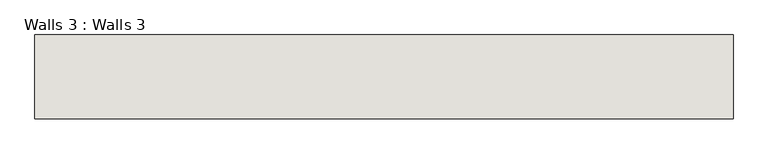
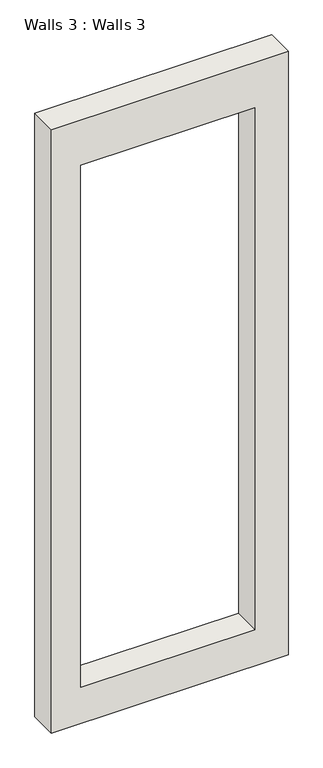
"""IFC4 building model written with IfcOpenShell, lengths in millimetres: wall geometry, Walls 3 : Walls 3."""

from ifc_helpers import new_model, si_unit, frame, origin, place, context, project, spatial, polyline, outline, extrude, source, transform, mapped, element, save


def walls_3_walls_3_431fb133(model_context):
    return source(origin(), model_context, "Body", "SweptSolid", [
        extrude(outline(polyline([(10430.0078921, -8481.8379698), (10430.0078921, -10760.3418199), (4290.5424183, -10760.3418199), (4290.5424183, -8481.8379698), (10430.0078921, -8481.8379698)]), holes=[polyline([(9967.4603713, -8801.0344883), (4658.3953761, -8801.0344883), (4658.3953761, -10477.4344883), (9967.4603713, -10477.4344883), (9967.4603713, -8801.0344883)])]), frame((0.0, -2901.4387205, 0.0), z_axis=(0.0, 1.0, 0.0), x_axis=(0.0, 0.0, 1.0)), (0.0, 0.0, 1.0), 272.9870857),
    ])


if __name__ == "__main__":
    model = new_model("IFC4")
    model_context = context("Model", 3, world=origin())
    ifc_project = project(units=[si_unit("LENGTHUNIT", "METRE", prefix="MILLI")], contexts=[model_context])
    site = spatial("IfcSite", under=ifc_project)
    building = spatial("IfcBuilding", under=site)
    placement = place(None, origin())
    walls_3_walls_3_shape = walls_3_walls_3_431fb133(model_context)
    element("IfcWall", 1, ObjectType="Walls 3 : Walls 3", at=placement, inside=building, context=model_context, shape_type="MappedRepresentation", body=[
        mapped(walls_3_walls_3_shape, transform((0.0, 0.0, 0.0), x_axis=(1.0, 0.0, 0.0), y_axis=(0.0, 1.0, 0.0), z_axis=(0.0, 0.0, 1.0))),
    ])
    save(model, "model.ifc")

# Revit data of these elements
# Element 1 (IfcWall, "Walls 3 : Walls 3")
#   Materials on its faces: "Default Wall"
# Materials
#   "Default Wall": colour RGB 128 128 128, transparency 0
